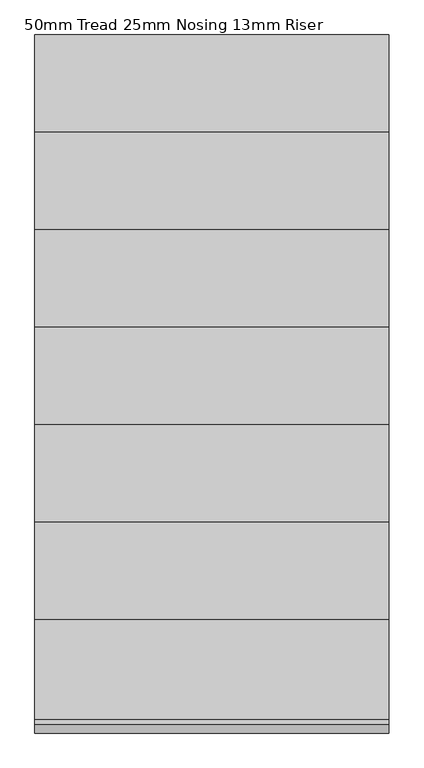
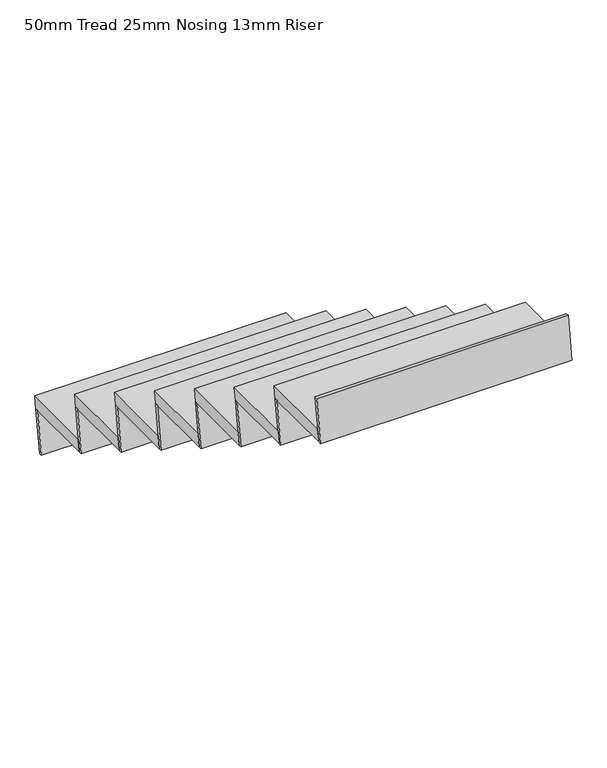
"""IFC4 building model written with IfcOpenShell, lengths in millimetres: stair flight geometry, 50mm Tread 25mm Nosing 13mm Riser."""

from ifc_helpers import new_model, si_unit, frame, origin, place, context, project, spatial, polyline, outline, extrude, source, transform, mapped, element, save


def stair_flight_50mm_tread_25mm_nosing_13mm_riser_daaaf0ad(model_context):
    return source(origin(), model_context, "Body", "SweptSolid", [
        extrude(outline(polyline([(10523.7482221, 1565.2173913), (10823.7482221, 1565.2173913), (10816.5607221, 1515.2173913), (10516.5607221, 1515.2173913), (10523.7482221, 1565.2173913)])), frame((-3440.2939506, 0.0, 0.0), z_axis=(1.0, 0.0, 0.0), x_axis=(0.0, 1.0, 0.0)), (0.0, 0.0, 1.0), 1000.0257812),
        extrude(outline(polyline([(10816.5607221, 1515.2173913), (10791.5607221, 1341.3043478), (10778.9322321, 1341.3043478), (10803.9322321, 1515.2173913), (10816.5607221, 1515.2173913)])), frame((-3440.2939506, 0.0, 0.0), z_axis=(1.0, 0.0, 0.0), x_axis=(0.0, 1.0, 0.0)), (0.0, 0.0, 1.0), 1000.0257813),
        extrude(outline(polyline([(10541.5607221, 1689.1304348), (10516.5607221, 1515.2173913), (10503.9322321, 1515.2173913), (10528.9322321, 1689.1304348), (10541.5607221, 1689.1304348)])), frame((-3440.2939506, 0.0, 0.0), z_axis=(1.0, 0.0, 0.0), x_axis=(0.0, 1.0, 0.0)), (0.0, 0.0, 1.0), 1000.0257813),
        extrude(outline(polyline([(10248.7482221, 1739.1304348), (10548.7482221, 1739.1304348), (10541.5607221, 1689.1304348), (10241.5607221, 1689.1304348), (10248.7482221, 1739.1304348)])), frame((-3440.2939506, 0.0, 0.0), z_axis=(1.0, 0.0, 0.0), x_axis=(0.0, 1.0, 0.0)), (0.0, 0.0, 1.0), 1000.0257813),
        extrude(outline(polyline([(10266.5607221, 1863.0434783), (10241.5607221, 1689.1304348), (10228.9322321, 1689.1304348), (10253.9322321, 1863.0434783), (10266.5607221, 1863.0434783)])), frame((-3440.2939506, 0.0, 0.0), z_axis=(1.0, 0.0, 0.0), x_axis=(0.0, 1.0, 0.0)), (0.0, 0.0, 1.0), 1000.0257813),
        extrude(outline(polyline([(9973.7482221, 1913.0434783), (10273.7482221, 1913.0434783), (10266.5607221, 1863.0434783), (9966.5607221, 1863.0434783), (9973.7482221, 1913.0434783)])), frame((-3440.2939506, 0.0, 0.0), z_axis=(1.0, 0.0, 0.0), x_axis=(0.0, 1.0, 0.0)), (0.0, 0.0, 1.0), 1000.0257813),
        extrude(outline(polyline([(9991.5607221, 2036.9565217), (9966.5607221, 1863.0434783), (9953.9322321, 1863.0434783), (9978.9322321, 2036.9565217), (9991.5607221, 2036.9565217)])), frame((-3440.2939506, 0.0, 0.0), z_axis=(1.0, 0.0, 0.0), x_axis=(0.0, 1.0, 0.0)), (0.0, 0.0, 1.0), 1000.0257813),
        extrude(outline(polyline([(9698.7482221, 2086.9565217), (9998.7482221, 2086.9565217), (9991.5607221, 2036.9565217), (9691.5607221, 2036.9565217), (9698.7482221, 2086.9565217)])), frame((-3440.2939506, 0.0, 0.0), z_axis=(1.0, 0.0, 0.0), x_axis=(0.0, 1.0, 0.0)), (0.0, 0.0, 1.0), 1000.0257813),
        extrude(outline(polyline([(9716.5607221, 2210.8695652), (9691.5607221, 2036.9565217), (9678.9322321, 2036.9565217), (9703.9322321, 2210.8695652), (9716.5607221, 2210.8695652)])), frame((-3440.2939506, 0.0, 0.0), z_axis=(1.0, 0.0, 0.0), x_axis=(0.0, 1.0, 0.0)), (0.0, 0.0, 1.0), 1000.0257813),
        extrude(outline(polyline([(9423.7482221, 2260.8695652), (9723.7482221, 2260.8695652), (9716.5607221, 2210.8695652), (9416.5607221, 2210.8695652), (9423.7482221, 2260.8695652)])), frame((-3440.2939506, 0.0, 0.0), z_axis=(1.0, 0.0, 0.0), x_axis=(0.0, 1.0, 0.0)), (0.0, 0.0, 1.0), 1000.0257813),
        extrude(outline(polyline([(9441.5607221, 2384.7826087), (9416.5607221, 2210.8695652), (9403.9322321, 2210.8695652), (9428.9322321, 2384.7826087), (9441.5607221, 2384.7826087)])), frame((-3440.2939506, 0.0, 0.0), z_axis=(1.0, 0.0, 0.0), x_axis=(0.0, 1.0, 0.0)), (0.0, 0.0, 1.0), 1000.0257813),
        extrude(outline(polyline([(9148.7482221, 2434.7826087), (9448.7482221, 2434.7826087), (9441.5607221, 2384.7826087), (9141.5607221, 2384.7826087), (9148.7482221, 2434.7826087)])), frame((-3440.2939506, 0.0, 0.0), z_axis=(1.0, 0.0, 0.0), x_axis=(0.0, 1.0, 0.0)), (0.0, 0.0, 1.0), 1000.0257813),
        extrude(outline(polyline([(9166.5607221, 2558.6956522), (9141.5607221, 2384.7826087), (9128.9322321, 2384.7826087), (9153.9322321, 2558.6956522), (9166.5607221, 2558.6956522)])), frame((-3440.2939506, 0.0, 0.0), z_axis=(1.0, 0.0, 0.0), x_axis=(0.0, 1.0, 0.0)), (0.0, 0.0, 1.0), 1000.0257813),
        extrude(outline(polyline([(8891.5607221, 2732.6086957), (8866.5607221, 2558.6956522), (8853.9322321, 2558.6956522), (8878.9322321, 2732.6086957), (8891.5607221, 2732.6086957)])), frame((-3440.2939506, 0.0, 0.0), z_axis=(1.0, 0.0, 0.0), x_axis=(0.0, 1.0, 0.0)), (0.0, 0.0, 1.0), 1000.0257813),
        extrude(outline(polyline([(8873.7482221, 2608.6956522), (9173.7482221, 2608.6956522), (9166.5607221, 2558.6956522), (8866.5607221, 2558.6956522), (8873.7482221, 2608.6956522)])), frame((-3440.2939506, 0.0, 0.0), z_axis=(1.0, 0.0, 0.0), x_axis=(0.0, 1.0, 0.0)), (0.0, 0.0, 1.0), 1000.0257812),
    ])


if __name__ == "__main__":
    model = new_model("IFC4")
    model_context = context("Model", 3, world=origin())
    ifc_project = project(units=[si_unit("LENGTHUNIT", "METRE", prefix="MILLI")], contexts=[model_context])
    site = spatial("IfcSite", under=ifc_project)
    building = spatial("IfcBuilding", under=site)
    placement = place(None, origin())
    stair_flight_50mm_tread_25mm_nosing_13mm_riser_shape = stair_flight_50mm_tread_25mm_nosing_13mm_riser_daaaf0ad(model_context)
    element("IfcStairFlight", 1, ObjectType="50mm Tread 25mm Nosing 13mm Riser", at=placement, inside=building, context=model_context, shape_type="MappedRepresentation", body=[
        mapped(stair_flight_50mm_tread_25mm_nosing_13mm_riser_shape, transform((0.0, 0.0, 0.0), x_axis=(1.0, 0.0, 0.0), y_axis=(0.0, 1.0, 0.0), z_axis=(0.0, 0.0, 1.0))),
    ])
    save(model, "model.ifc")
